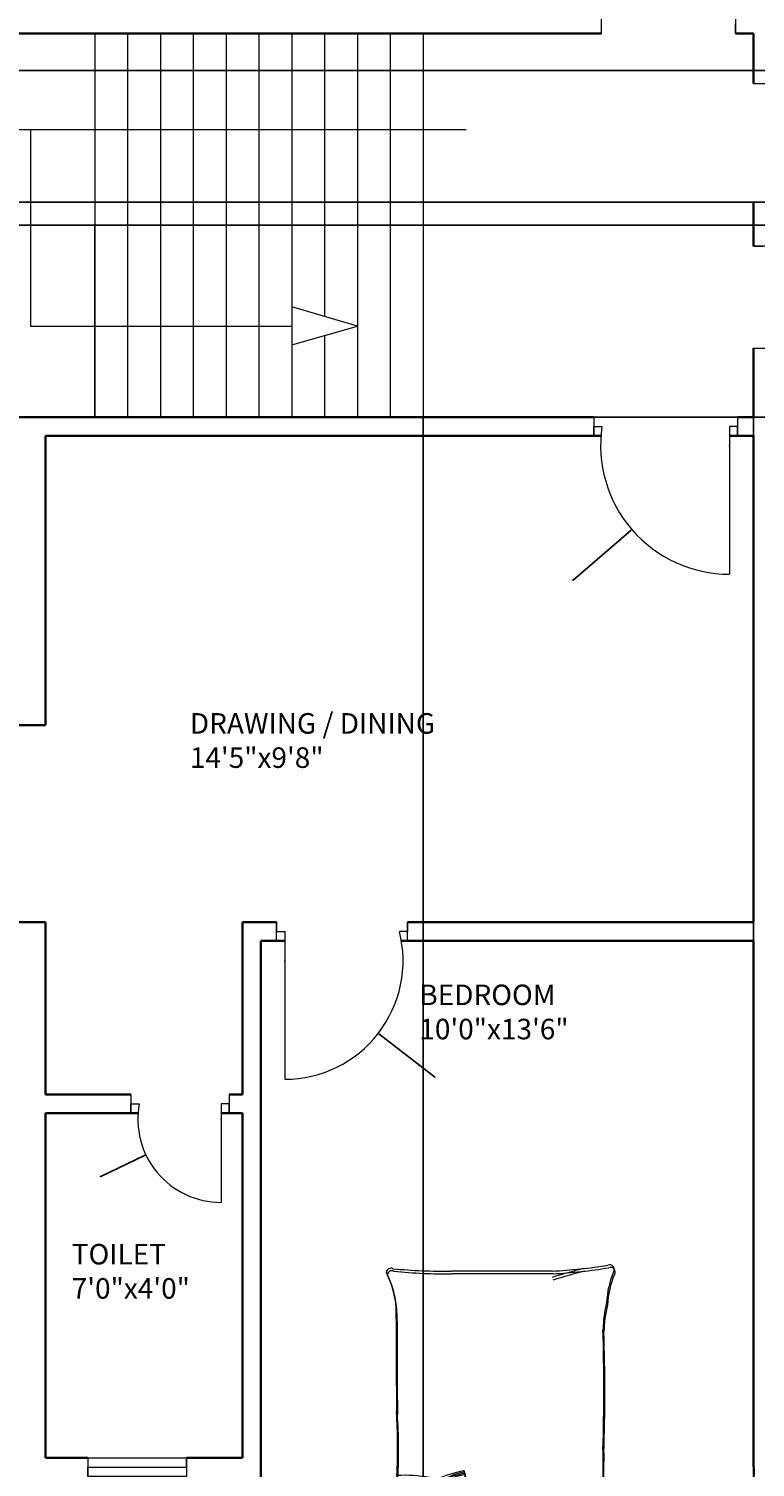
# Model space of a CAD drawing. Units: inches. Extents: x 1937 to 2996, y 1402 to 2323.
# Tile 4 of 10: x 2466 to 2643, y 1594 to 1944. Entities that reach past the tile are written whole.
import ezdxf

# ---------------------------------------------------------------- set-up
doc = ezdxf.new("R2010")
doc.units = ezdxf.units.IN
for name, color, linetype, lineweight in [('A-ANNO-DIMS', 2, 'Continuous', 18), ('A-AREA-IDEN', 7, 'Continuous', 18), ('A-DOOR', 11, 'Continuous', 18), ('A-FLOR-STRS', 81, 'Continuous', 18), ('A-FURN', 8, 'Continuous', 13), ('A-GLAZ', 141, 'Continuous', 18), ('A-WALL', 7, 'Continuous', 35)]:
    doc.layers.add(name, color=color, linetype=linetype, lineweight=lineweight)
doc.styles.get("Standard").update_dxf_attribs({"font": 'arial.ttf'})
doc.dimstyles.get("Standard").update_dxf_attribs({"dimtxt": 0.18, "dimasz": 0.18, "dimexe": 0.18, "dimexo": 0.0625, "dimgap": 0.09, "dimtad": 0, "dimtih": 1, "dimtoh": 1, "dimdec": 4, "dimzin": 0, "dimdsep": 46, "dimtxsty": 'Standard', "dimcen": 0.09, "dimadec": 0, "dimazin": 0, "dimtfac": 1, "dimtdec": 4, "dimtofl": 0, "dimtmove": 0, "dimatfit": 3, "dimfxl": 1, "dimtolj": 1, "dimtzin": 0, "dimarcsym": 0})

# ---------------------------------------------------------------- blocks, each defined once
blk = doc.blocks.new('BED-DOUBLE')
for p, q in [((-24.01, -18.11), (-24.01, 0)), ((-24.01, -18.11), (-24.01, 0)), ((-24.01, 0), (24.01, 0)), ((23.78, 0), (23.78, -26.61)), ((23.78, 0), (23.78, -26.61)), ((24.01, 0), (24.01, -0.64)), ((-24.01, -1.53), (23.78, -1.53)), ((-24.01, -1.53), (23.78, -1.53)), ((-23.78, -18.75), (-23.78, -0.64)), ((-23.78, -18.75), (-23.78, -0.64)), ((-23.78, -2.17), (24.01, -2.17)), ((-23.78, -2.17), (24.01, -2.17)), ((-23.59, -3.34), (-19.3, -3.01)), ((-23.59, -3.34), (-19.31, -3.01)), ((-23.59, -3.32), (-23.01, -6.5)), ((-23.59, -3.32), (-23.01, -6.5)), ((-19.31, -3.01), (-19.2, -3.03)), ((-19.3, -3.01), (-19.2, -3.03)), ((-19.2, -3.03), (-15.38, -3.32)), ((-19.2, -3.03), (-15.38, -3.32)), ((-15.38, -3.32), (-9.88, -4.33)), ((-15.38, -3.32), (-9.88, -4.33)), ((-12.63, -3.75), (-10.61, -3.03)), ((-12.63, -3.75), (-10.61, -3.03)), ((-10.61, -3.03), (-7.71, -2.3)), ((-10.61, -3.03), (-7.71, -2.3)), ((-10.38, -3.67), (-7.49, -2.94)), ((-10.38, -3.67), (-7.49, -2.94)), ((-7.71, -2.3), (-7.39, -2.3)), ((-7.71, -2.3), (-7.39, -2.3)), ((-7.49, -2.94), (-7.16, -2.94)), ((-7.49, -2.94), (-7.16, -2.94)), ((-7.39, -2.3), (-2.95, -2.45)), ((-7.39, -2.3), (-2.95, -2.45)), ((-7.16, -2.94), (-2.72, -3.09)), ((-7.16, -2.94), (-2.72, -3.09)), ((-2.95, -2.45), (-1.5, -1.87)), ((-2.95, -2.45), (-1.5, -1.87)), ((-2.72, -3.09), (-1.27, -2.51)), ((-2.72, -3.09), (-1.27, -2.51)), ((-1.5, -1.87), (-0.92, -7.22)), ((-1.5, -1.87), (-0.92, -7.22)), ((-1.27, -2.51), (-0.7, -7.86)), ((-1.27, -2.51), (-0.7, -7.86)), ((0.49, -2.49), (0.25, -7.87)), ((0.49, -2.49), (0.25, -7.87)), ((0.72, -3.13), (0.48, -8.51)), ((0.72, -3.13), (0.48, -8.51)), ((1.97, -2.98), (0.49, -2.49)), ((1.97, -2.98), (0.49, -2.49)), ((2.2, -3.62), (0.72, -3.13)), ((2.2, -3.62), (0.72, -3.13)), ((6.4, -2.56), (1.97, -2.98)), ((6.4, -2.56), (1.97, -2.98)), ((6.63, -3.2), (2.2, -3.62)), ((6.63, -3.2), (2.2, -3.62)), ((6.72, -2.54), (6.4, -2.56)), ((6.72, -2.54), (6.4, -2.56)), ((6.95, -3.18), (6.63, -3.2)), ((6.95, -3.18), (6.63, -3.2)), ((9.65, -3.08), (6.72, -2.54)), ((9.65, -3.08), (6.72, -2.54)), ((9.88, -3.72), (6.95, -3.18)), ((9.88, -3.72), (6.95, -3.18)), ((14.43, -3.07), (9.01, -4.42)), ((14.43, -3.07), (9.01, -4.42)), ((11.72, -3.67), (9.65, -3.08)), ((11.72, -3.67), (9.65, -3.08)), ((18.23, -2.54), (14.43, -3.07)), ((18.23, -2.54), (14.43, -3.07)), ((18.46, -3.18), (14.66, -3.71)), ((18.46, -3.18), (14.66, -3.71)), ((22.63, -2.56), (17.23, -2.46)), ((17.23, -2.46), (18.23, -2.54)), ((22.63, -2.56), (17.23, -2.46)), ((17.23, -2.46), (18.23, -2.54)), ((22.86, -3.2), (17.45, -3.1)), ((17.45, -3.1), (18.46, -3.18)), ((22.86, -3.2), (17.45, -3.1)), ((17.45, -3.1), (18.46, -3.18)), ((22.63, -2.56), (22.25, -5.77)), ((22.63, -2.56), (22.25, -5.77)), ((22.86, -3.2), (22.48, -6.41)), ((22.86, -3.2), (22.48, -6.41)), ((24.01, -0.64), (24.01, -27.25)), ((24.01, -0.64), (24.01, -27.25)), ((-23.01, -6.5), (-23.45, -9.1)), ((-23.01, -6.5), (-23.45, -9.1)), ((-23.36, -3.98), (-19.08, -3.65)), ((-23.36, -3.98), (-19.08, -3.65)), ((-23.36, -3.96), (-22.78, -7.14)), ((-23.36, -3.96), (-22.78, -7.14)), ((-22.43, -8.96), (-21.42, -6.21)), ((-22.43, -8.96), (-21.42, -6.21)), ((-22.21, -9.59), (-21.19, -6.85)), ((-22.2, -9.59), (-21.19, -6.85)), ((-19.08, -3.65), (-18.97, -3.67)), ((-19.08, -3.65), (-18.97, -3.67)), ((-18.97, -3.67), (-15.15, -3.96)), ((-18.97, -3.67), (-15.15, -3.96)), ((-15.15, -3.96), (-9.65, -4.97)), ((-15.15, -3.96), (-9.65, -4.97)), ((-12.4, -4.39), (-10.38, -3.67)), ((-12.4, -4.39), (-10.38, -3.67)), ((14.66, -3.71), (9.24, -5.06)), ((14.66, -3.71), (9.24, -5.06)), ((11.94, -4.31), (9.88, -3.72)), ((11.94, -4.31), (9.88, -3.72)), ((21.83, -8.26), (20.64, -5.58)), ((21.82, -8.26), (20.64, -5.58)), ((22.05, -8.9), (20.87, -6.22)), ((22.05, -8.9), (20.87, -6.22)), ((22.25, -5.77), (22.84, -8.34)), ((22.25, -5.77), (22.84, -8.34)), ((22.48, -6.41), (23.07, -8.98)), ((22.48, -6.41), (23.07, -8.98)), ((-23.45, -9.1), (-22.87, -10.11)), ((-23.45, -9.1), (-22.87, -10.11)), ((-22.78, -7.14), (-23.22, -9.74)), ((-22.78, -7.14), (-23.22, -9.74)), ((-23.22, -9.74), (-22.64, -10.75)), ((-23.22, -9.74), (-22.64, -10.75)), ((-23.01, -12.57), (-22.43, -8.96)), ((-23.01, -12.57), (-22.43, -8.96)), ((-22.78, -13.21), (-22.2, -9.59)), ((-22.78, -13.21), (-22.21, -9.59)), ((-0.92, -7.22), (-0.35, -10.4)), ((-0.92, -7.22), (-0.35, -10.4)), ((-0.7, -7.86), (-0.12, -11.04)), ((-0.7, -7.86), (-0.12, -11.04)), ((-0.35, -10.4), (-0.35, -11.7)), ((-0.35, -10.4), (-0.35, -11.7)), ((0.25, -7.87), (-0.13, -11.08)), ((0.25, -7.87), (-0.13, -11.08)), ((0.48, -8.51), (0.1, -11.72)), ((0.48, -8.51), (0.1, -11.72)), ((22.63, -11.83), (21.82, -8.26)), ((22.63, -11.83), (21.83, -8.26)), ((22.86, -12.47), (22.05, -8.9)), ((22.86, -12.47), (22.05, -8.9)), ((22.84, -8.34), (22.33, -9.38)), ((22.84, -8.34), (22.33, -9.38)), ((23.07, -8.98), (22.56, -10.02)), ((23.07, -8.98), (22.56, -10.02)), ((-22.72, -14.16), (-23.01, -12.57)), ((-22.72, -14.16), (-23.01, -12.57)), ((-22.49, -14.8), (-22.78, -13.21)), ((-22.49, -14.8), (-22.78, -13.21)), ((-0.35, -11.7), (-0.92, -13.58)), ((-0.35, -11.7), (-0.92, -13.58)), ((-0.92, -13.58), (-0.92, -16.26)), ((-0.92, -13.58), (-0.92, -16.26)), ((-0.12, -12.34), (-0.7, -14.22)), ((-0.12, -12.34), (-0.7, -14.22)), ((-0.13, -11.08), (-0.05, -12.38)), ((-0.13, -11.08), (-0.05, -12.38)), ((-0.12, -11.04), (-0.12, -12.34)), ((-0.12, -11.04), (-0.12, -12.34)), ((-0.05, -12.38), (0.65, -14.22)), ((-0.05, -12.38), (0.65, -14.22)), ((0.1, -11.72), (0.18, -13.02)), ((0.1, -11.72), (0.18, -13.02)), ((0.18, -13.02), (0.87, -14.86)), ((0.18, -13.02), (0.87, -14.86)), ((22.44, -13.43), (22.63, -11.83)), ((22.44, -13.43), (22.63, -11.83)), ((23.21, -16.57), (22.44, -13.43)), ((23.21, -16.57), (22.44, -13.43)), ((22.67, -14.07), (22.86, -12.47)), ((22.67, -14.07), (22.86, -12.47)), ((-23.3, -17.34), (-22.72, -14.16)), ((-23.3, -17.34), (-22.72, -14.16)), ((-18.2, -16.62), (-23.3, -17.34)), ((-18.2, -16.62), (-23.3, -17.34)), ((-23.07, -17.98), (-22.49, -14.8)), ((-23.07, -17.98), (-22.49, -14.8)), ((-17.98, -17.26), (-23.07, -17.98)), ((-17.98, -17.26), (-23.07, -17.98)), ((-21.1, -15.63), (-17.07, -16.3)), ((-21.1, -15.63), (-17.07, -16.3)), ((-20.87, -16.27), (-16.84, -16.93)), ((-20.87, -16.27), (-16.84, -16.93)), ((-17.07, -16.3), (-18.2, -16.62)), ((-17.07, -16.3), (-18.2, -16.62)), ((-16.84, -16.93), (-17.98, -17.26)), ((-16.84, -16.93), (-17.98, -17.26)), ((-17.07, -16.3), (-10.06, -16.73)), ((-17.07, -16.3), (-10.06, -16.73)), ((-16.84, -16.93), (-9.83, -17.37)), ((-16.84, -16.93), (-9.83, -17.37)), ((-10.06, -16.73), (-8.1, -16.17)), ((-10.06, -16.73), (-8.1, -16.17)), ((-9.83, -17.37), (-7.87, -16.81)), ((-9.83, -17.37), (-7.87, -16.81)), ((-8.1, -16.17), (-2.97, -16.57)), ((-8.1, -16.17), (-2.97, -16.57)), ((-7.87, -16.81), (-2.74, -17.21)), ((-7.87, -16.81), (-2.74, -17.21)), ((-3.38, -16.26), (-6.53, -15.17)), ((-3.38, -16.26), (-6.53, -15.17)), ((-3.15, -16.9), (-6.3, -15.81)), ((-3.15, -16.9), (-6.3, -15.81)), ((-0.92, -16.26), (-3.38, -16.26)), ((-0.92, -16.26), (-3.38, -16.26)), ((-0.7, -16.9), (-3.15, -16.9)), ((-0.7, -16.9), (-3.15, -16.9)), ((-0.7, -14.22), (-0.7, -16.9)), ((-0.7, -14.22), (-0.7, -16.9)), ((0.65, -14.22), (0.81, -16.89)), ((0.65, -14.22), (0.81, -16.89)), ((0.81, -16.89), (3.27, -16.74)), ((0.81, -16.89), (3.27, -16.74)), ((0.87, -14.86), (1.04, -17.53)), ((0.87, -14.86), (1.04, -17.53)), ((1.04, -17.53), (3.49, -17.38)), ((1.04, -17.53), (3.49, -17.38)), ((2.77, -17.38), (6.97, -23.88)), ((2.77, -17.38), (6.96, -23.88)), ((3.27, -16.74), (6.34, -15.45)), ((3.27, -16.74), (6.34, -15.45)), ((3.49, -17.38), (6.56, -16.09)), ((3.49, -17.38), (6.56, -16.09)), ((13.16, -20.32), (4.82, -17.38)), ((13.16, -20.32), (4.82, -17.38)), ((5.08, -15.63), (9.11, -16.3)), ((5.08, -15.63), (9.11, -16.3)), ((5.31, -16.27), (9.34, -16.93)), ((5.31, -16.27), (9.34, -16.93)), ((9.11, -16.3), (16.12, -16.73)), ((9.11, -16.3), (16.12, -16.73)), ((9.34, -16.93), (16.35, -17.37)), ((9.34, -16.93), (16.35, -17.37)), ((16.12, -16.73), (18.08, -16.17)), ((16.12, -16.73), (18.08, -16.17)), ((16.35, -17.37), (18.31, -16.81)), ((16.35, -17.37), (18.31, -16.81)), ((18.08, -16.17), (23.21, -16.57)), ((18.08, -16.17), (23.21, -16.57)), ((18.31, -16.81), (23.44, -17.21)), ((18.31, -16.81), (23.44, -17.21)), ((23.44, -17.21), (22.67, -14.07)), ((23.44, -17.21), (22.67, -14.07)), ((3, -18.02), (7.19, -24.52)), ((3, -18.02), (7.19, -24.52)), ((13.39, -20.96), (5.05, -18.02)), ((13.39, -20.96), (5.05, -18.02)), ((18.74, -22.33), (13.16, -20.32)), ((18.74, -22.33), (13.16, -20.32)), ((18.96, -22.97), (13.39, -20.96)), ((18.96, -22.97), (13.39, -20.96)), ((6.96, -23.88), (8.67, -28.37)), ((6.97, -23.88), (8.67, -28.37)), ((7.19, -24.52), (8.9, -29)), ((7.19, -24.52), (8.9, -29)), ((21.68, -24.5), (18.74, -22.33)), ((21.68, -24.5), (18.74, -22.33)), ((21.91, -25.13), (18.96, -22.97)), ((21.91, -25.13), (18.96, -22.97)), ((25.38, -27.75), (21.68, -24.5)), ((25.38, -27.75), (21.68, -24.5)), ((25.61, -28.39), (21.91, -25.13)), ((25.61, -28.39), (21.91, -25.13)), ((23.85, -28.37), (25.38, -27.75)), ((23.85, -28.37), (25.38, -27.75)), ((25.46, -29.49), (25.38, -27.75, 3.87)), ((25.46, -29.49), (25.38, -27.75, 3.87)), ((8.67, -28.37), (8.98, -30.38)), ((8.67, -28.37), (8.98, -30.38)), ((8.9, -29), (9.21, -31.02)), ((8.9, -29), (9.21, -31.02)), ((8.98, -30.38), (11.46, -29.76)), ((8.98, -30.38), (11.46, -29.76)), ((9.21, -31.02), (11.68, -30.4)), ((9.21, -31.02), (11.68, -30.4)), ((11.46, -29.76), (13.47, -28.83)), ((11.46, -29.76), (13.47, -28.83)), ((11.68, -30.4), (13.7, -29.47)), ((11.68, -30.4), (13.7, -29.47)), ((13.47, -28.83), (16.88, -28.37)), ((13.47, -28.83), (16.88, -28.37)), ((13.7, -29.47), (17.11, -29)), ((13.7, -29.47), (17.1, -29)), ((16.88, -28.37), (20.75, -28.06)), ((16.88, -28.37), (20.75, -28.06)), ((17.1, -29), (20.98, -28.69)), ((17.11, -29), (20.98, -28.69)), ((20.75, -28.06), (23.85, -28.37)), ((20.75, -28.06), (23.85, -28.37)), ((20.98, -28.69), (24.07, -29)), ((20.98, -28.69), (24.07, -29)), ((24.07, -29), (25.61, -28.39)), ((24.07, -29), (25.61, -28.39)), ((25.69, -30.13), (25.61, -28.39, 3.87)), ((25.69, -30.13), (25.61, -28.39, 3.87)), ((-12.42, -79.25), (12.19, -79.25)), ((-12.42, -79.25), (12.19, -79.25)), ((-12.19, -79.88), (12.42, -79.88)), ((-12.19, -79.88), (12.42, -79.88))]:
    blk.add_line(p, q)
for centre, radius, start, end in [((-6.13, -182.05), 164.97, 86.0865, 96.7821), ((-6.13, -182.05), 164.97, 86.0865, 96.7821), ((57.68, -20.1), 83.31, 178.7218, 185.604), ((57.68, -20.1), 83.31, 178.7218, 185.604), ((57.91, -20.74), 83.31, 178.7218, 185.604), ((57.91, -20.74), 83.31, 178.7218, 185.604), ((-5.9, -182.69), 164.97, 86.0865, 96.7821), ((-5.9, -182.69), 164.97, 86.0865, 96.7821), ((-9.73, -156.32), 129.02, 81.7845, 96.9006), ((-9.73, -156.32), 129.02, 81.7845, 96.9006), ((-9.5, -156.96), 129.02, 81.7845, 96.9006), ((-9.5, -156.96), 129.02, 81.7845, 96.9006), ((-194.79, -31.17), 170.11, 358.4762, 1.0082), ((-194.79, -31.17), 170.11, 358.4762, 1.0082), ((-194.56, -31.81), 170.11, 358.4762, 1.0082), ((-194.56, -31.81), 170.11, 358.4762, 1.0082), ((9.15, -30.44), 0.185, 160.2464, 271.1377), ((9.15, -30.44), 0.185, 160.2464, 271.1377), ((3.67, -1.48), 29.65, 280.6617, 289.8806), ((3.67, -1.48), 29.65, 280.6617, 289.8806), ((9.38, -31.08), 0.185, 160.2464, 271.1377), ((9.38, -31.08), 0.185, 160.2464, 271.1377), ((3.9, -2.12), 29.65, 280.6617, 289.8806), ((3.9, -2.12), 29.65, 280.6617, 289.8806), ((16.26, -35.07), 6.22, 78.6608, 113.7384), ((16.26, -35.07), 6.22, 78.6608, 113.7384), ((16.49, -35.71), 6.22, 78.6608, 113.7384), ((16.49, -35.71), 6.22, 78.6608, 113.7384), ((23.84, 6.66), 36.18, 259.8763, 272.5657), ((23.84, 6.66), 36.18, 259.8763, 272.5657), ((24.07, 6.02), 36.18, 259.8763, 272.5657), ((24.07, 6.02), 36.18, 259.8763, 272.5657), ((154.78, -36.32), 129.5, 176.9791, 183.8365), ((154.78, -36.32), 129.5, 176.9791, 183.8365), ((155.01, -36.95), 129.5, 176.9791, 183.8365), ((155.01, -36.95), 129.5, 176.9791, 183.8365), ((457.34, -50.61), 482.31, 178.2277, 181.7185), ((457.34, -50.61), 482.31, 178.2277, 181.7185), ((457.57, -51.25), 482.31, 178.2277, 181.7185), ((457.57, -51.25), 482.31, 178.2277, 181.7185), ((-4536.23, -67.82), 4561.86, 0.00217, 0.28689), ((-4536.23, -67.82), 4561.86, 0.00217, 0.28689), ((-4536, -68.46), 4561.86, 0.00217, 0.28689), ((-4536, -68.46), 4561.86, 0.00217, 0.28689), ((-54.38, -64.52), 29.63, 346.0648, 358.9113), ((-54.38, -64.52), 29.63, 346.0648, 358.9113), ((-54.16, -65.15), 29.63, 346.0648, 358.9113), ((-54.16, -65.15), 29.63, 346.0648, 358.9113), ((48.67, -68.67), 23.07, 177.4714, 206.4681), ((48.67, -68.67), 23.07, 177.4714, 206.4681), ((48.9, -69.31), 23.07, 177.4714, 206.4681), ((48.9, -69.31), 23.07, 177.4714, 206.4681), ((-49.14, -70.28), 23.56, 337.9751, 356.652), ((-49.14, -70.28), 23.56, 337.9751, 356.652), ((-48.92, -70.91), 23.56, 337.9751, 356.652), ((-48.92, -70.91), 23.56, 337.9751, 356.652), ((-26.4, -79.72), 1.09, 146.1736, 293.4781), ((-26.4, -79.72), 1.09, 146.1736, 293.4781), ((-26.17, -80.36), 1.09, 146.1736, 293.4781), ((-26.17, -80.36), 1.09, 146.1736, 293.4781), ((-6.06, -200.84), 121.76, 92.9958, 99.4091), ((-6.06, -200.84), 121.76, 92.9958, 99.4091), ((-5.83, -201.48), 121.76, 92.9958, 99.4091), ((-5.83, -201.48), 121.76, 92.9958, 99.4091), ((-44.71, 23.71), 106.46, 283.3832, 287.7053), ((-44.71, 23.71), 106.46, 283.3832, 287.7053), ((-44.48, 23.07), 106.46, 283.3832, 287.7053), ((-44.48, 23.07), 106.46, 283.3832, 287.7053), ((13.67, -212.28), 133.04, 84.4998, 90.6351), ((13.67, -212.28), 133.04, 84.4998, 90.6351), ((13.9, -212.92), 133.04, 84.4998, 90.6351), ((13.9, -212.92), 133.04, 84.4998, 90.6351), ((26.93, -78.87), 1.1, 242.6588, 356.02), ((26.93, -78.87), 1.1, 242.6588, 356.02), ((27.15, -79.51), 1.1, 242.6588, 356.02), ((27.15, -79.51), 1.1, 242.6588, 356.02)]:
    blk.add_arc(centre, radius, start, end)
blk = doc.blocks.new('WINDOW-24IN')
for p, q in [((0, -2.25), (0, 2.25)), ((0, 2.25), (0, 0)), ((24, 2.25), (0, 2.25)), ((0, 0), (24, 0)), ((24, -2.25), (24, 2.25)), ((24, 0), (24, -2.25)), ((0, -2.25), (24, -2.25))]:
    blk.add_line(p, q)
blk = doc.blocks.new('*D23')
at = {"layer": 'A-ANNO-DIMS', "color": 0, "lineweight": -2, "transparency": 16777216}
for p, q in [((2010.65, 1769.24), (2010.65, 1508.98)), ((2924.15, 1769.24), (2924.15, 1508.98)), ((2010.83, 1509.16), (2467, 1509.16)), ((2923.97, 1509.16), (2467.79, 1509.16))]:
    blk.add_line(p, q, dxfattribs=at)
at = {"layer": 'A-ANNO-DIMS', "color": 0, "transparency": 16777216}
for points in [[(2010.83, 1509.19), (2010.83, 1509.13), (2010.65, 1509.16)], [(2923.97, 1509.19), (2923.97, 1509.13), (2924.15, 1509.16)]]:
    blk.add_solid(points, dxfattribs=at)
at = {"layer": 'Defpoints', "color": 0, "transparency": 16777216}
for p in [(2010.65, 1769.31), (2924.15, 1769.31), (2924.15, 1509.16)]:
    blk.add_point(p, dxfattribs=at)
at = {"layer": 'A-ANNO-DIMS', "color": 0, "transparency": 16777216, "insert": (2467.4, 1509.16), "char_height": 0.18, "attachment_point": 5}
blk.add_mtext('\\A1;913.5', dxfattribs=at)
blk = doc.blocks.new('*D34')
at = {"layer": 'A-ANNO-DIMS', "color": 0, "lineweight": -2, "transparency": 16777216}
for p, q in [((2350.61, 1849.24), (2350.61, 1508.98)), ((2561.65, 1849.24), (2561.65, 1508.98)), ((2350.79, 1509.16), (2455.66, 1509.16)), ((2561.47, 1509.16), (2456.59, 1509.16))]:
    blk.add_line(p, q, dxfattribs=at)
at = {"layer": 'A-ANNO-DIMS', "color": 0, "transparency": 16777216}
for points in [[(2350.79, 1509.19), (2350.79, 1509.13), (2350.61, 1509.16)], [(2561.47, 1509.19), (2561.47, 1509.13), (2561.65, 1509.16)]]:
    blk.add_solid(points, dxfattribs=at)
at = {"layer": 'Defpoints', "color": 0, "transparency": 16777216}
for p in [(2350.61, 1849.31), (2561.65, 1849.31), (2561.65, 1509.16)]:
    blk.add_point(p, dxfattribs=at)
at = {"layer": 'A-ANNO-DIMS', "color": 0, "transparency": 16777216, "insert": (2456.13, 1509.16), "char_height": 0.18, "attachment_point": 5}
blk.add_mtext('\\A1;211.04', dxfattribs=at)
blk = doc.blocks.new('*D35')
at = {"layer": 'A-ANNO-DIMS', "color": 0, "lineweight": -2, "transparency": 16777216}
for p, q in [((2561.65, 1849.24), (2561.65, 1508.98)), ((2642.15, 1849.24), (2642.15, 1508.98)), ((2561.83, 1509.16), (2601.57, 1509.16)), ((2641.97, 1509.16), (2602.22, 1509.16))]:
    blk.add_line(p, q, dxfattribs=at)
at = {"layer": 'A-ANNO-DIMS', "color": 0, "transparency": 16777216}
for points in [[(2561.83, 1509.19), (2561.83, 1509.13), (2561.65, 1509.16)], [(2641.97, 1509.19), (2641.97, 1509.13), (2642.15, 1509.16)]]:
    blk.add_solid(points, dxfattribs=at)
at = {"layer": 'Defpoints', "color": 0, "transparency": 16777216}
for p in [(2561.65, 1849.31), (2642.15, 1849.31), (2642.15, 1509.16)]:
    blk.add_point(p, dxfattribs=at)
at = {"layer": 'A-ANNO-DIMS', "color": 0, "transparency": 16777216, "insert": (2601.9, 1509.16), "char_height": 0.18, "attachment_point": 5}
blk.add_mtext('\\A1;80.5', dxfattribs=at)
blk = doc.blocks.new('*D37')
at = {"layer": 'A-ANNO-DIMS', "color": 0, "lineweight": -2, "transparency": 16777216}
for p, q in [((2455.84, 1896.06), (2970.48, 1896.06)), ((2970.3, 1895.88), (2970.3, 1872.86)), ((2970.3, 1849.49), (2970.3, 1872.5)), ((2455.84, 1849.31), (2970.48, 1849.31))]:
    blk.add_line(p, q, dxfattribs=at)
at = {"layer": 'A-ANNO-DIMS', "color": 0, "transparency": 16777216}
for points in [[(2970.27, 1895.88), (2970.33, 1895.88), (2970.3, 1896.06)], [(2970.27, 1849.49), (2970.33, 1849.49), (2970.3, 1849.31)]]:
    blk.add_solid(points, dxfattribs=at)
at = {"layer": 'Defpoints', "color": 0, "transparency": 16777216}
for p in [(2455.77, 1896.06), (2455.77, 1849.31), (2970.3, 1849.31)]:
    blk.add_point(p, dxfattribs=at)
at = {"layer": 'A-ANNO-DIMS', "color": 0, "transparency": 16777216, "insert": (2970.3, 1872.68), "char_height": 0.18, "attachment_point": 5}
blk.add_mtext('\\A1;46.75', dxfattribs=at)
blk = doc.blocks.new('*D50')
at = {"layer": 'A-ANNO-DIMS', "color": 0, "lineweight": -2, "transparency": 16777216}
for p, q in [((2292.71, 1933.76), (2970.48, 1933.76)), ((2970.3, 1933.58), (2970.3, 1917.9)), ((2970.3, 1901.85), (2970.3, 1917.53)), ((2292.71, 1901.67), (2970.48, 1901.67))]:
    blk.add_line(p, q, dxfattribs=at)
at = {"layer": 'A-ANNO-DIMS', "color": 0, "transparency": 16777216}
for points in [[(2970.27, 1933.58), (2970.33, 1933.58), (2970.3, 1933.76)], [(2970.27, 1901.85), (2970.33, 1901.85), (2970.3, 1901.67)]]:
    blk.add_solid(points, dxfattribs=at)
at = {"layer": 'Defpoints', "color": 0, "transparency": 16777216}
for p in [(2292.65, 1933.76), (2970.3, 1933.76), (2292.65, 1901.67)]:
    blk.add_point(p, dxfattribs=at)
at = {"layer": 'A-ANNO-DIMS', "color": 0, "transparency": 16777216, "insert": (2970.3, 1917.71), "char_height": 0.18, "attachment_point": 5}
blk.add_mtext('\\A1;32.085', dxfattribs=at)
blk = doc.blocks.new('*D56')
at = {"layer": 'A-ANNO-DIMS', "color": 0, "lineweight": -2, "transparency": 16777216}
for p, q in [((2636.21, 1842.45), (2636.39, 1842.45)), ((2636.3, 1842.36), (2636.3, 1842.54)), ((2598.27, 1809.64), (2612.4, 1821.83)), ((2598.09, 1809.64), (2598.27, 1809.64))]:
    blk.add_line(p, q, dxfattribs=at)
at = {"layer": 'A-ANNO-DIMS', "color": 0, "transparency": 16777216}
blk.add_solid([(2612.38, 1821.85), (2612.42, 1821.8), (2612.53, 1821.94)], dxfattribs=at)
at = {"layer": 'Defpoints', "color": 0, "transparency": 16777216}
for p in [(2636.3, 1842.45), (2612.53, 1821.94)]:
    blk.add_point(p, dxfattribs=at)
at = {"layer": 'A-ANNO-DIMS', "color": 0, "transparency": 16777216, "insert": (2597.54, 1809.64), "char_height": 0.18, "attachment_point": 5}
blk.add_mtext('\\A1;R31.394', dxfattribs=at)
blk = doc.blocks.new('*D64')
at = {"layer": 'A-ANNO-DIMS', "color": 0, "lineweight": -2, "transparency": 16777216}
for p, q in [((2527.87, 1716.88), (2528.05, 1716.88)), ((2527.96, 1716.79), (2527.96, 1716.97)), ((2564.41, 1688.62), (2550.88, 1699.11)), ((2564.59, 1688.62), (2564.41, 1688.62))]:
    blk.add_line(p, q, dxfattribs=at)
at = {"layer": 'A-ANNO-DIMS', "color": 0, "transparency": 16777216}
blk.add_solid([(2550.9, 1699.13), (2550.86, 1699.08), (2550.74, 1699.22)], dxfattribs=at)
at = {"layer": 'Defpoints', "color": 0, "transparency": 16777216}
for p in [(2527.96, 1716.88), (2550.74, 1699.22)]:
    blk.add_point(p, dxfattribs=at)
at = {"layer": 'A-ANNO-DIMS', "color": 0, "transparency": 16777216, "insert": (2565.14, 1688.62), "char_height": 0.18, "attachment_point": 5}
blk.add_mtext('\\A1;R28.823', dxfattribs=at)
blk = doc.blocks.new('*D86')
at = {"layer": 'A-ANNO-DIMS', "color": 0, "lineweight": -2, "transparency": 16777216}
for p, q in [((2512.36, 1678.36), (2512.54, 1678.36)), ((2512.45, 1678.27), (2512.45, 1678.45)), ((2483.12, 1664.39), (2493.96, 1669.55)), ((2482.94, 1664.39), (2483.12, 1664.39))]:
    blk.add_line(p, q, dxfattribs=at)
at = {"layer": 'A-ANNO-DIMS', "color": 0, "transparency": 16777216}
blk.add_solid([(2493.94, 1669.58), (2493.97, 1669.52), (2494.12, 1669.63)], dxfattribs=at)
at = {"layer": 'Defpoints', "color": 0, "transparency": 16777216}
for p in [(2512.45, 1678.36), (2494.12, 1669.63)]:
    blk.add_point(p, dxfattribs=at)
at = {"layer": 'A-ANNO-DIMS', "color": 0, "transparency": 16777216, "insert": (2482.39, 1664.39), "char_height": 0.18, "attachment_point": 5}
blk.add_mtext('\\A1;R20.303', dxfattribs=at)

msp = doc.modelspace()

# ---------------------------------------------------------------- linework, layer by layer
at = {"layer": 'A-DOOR'}
for p, q in [((2605.163, 1942.8061), (2605.163, 1947.3061)), ((2637.7727, 1947.3061), (2637.7727, 1942.8061)), ((2637.7727, 1942.8061), (2637.7727, 1945.0561)), ((2642.1473, 1930.5712), (2646.6473, 1930.5712)), ((2646.6473, 1901.7001), (2642.1473, 1901.7001)), ((2642.1473, 1901.7001), (2644.3973, 1901.7001)), ((2646.6473, 1890.9534), (2642.1473, 1890.9534)), ((2642.1473, 1890.9534), (2644.3973, 1890.9534)), ((2642.1473, 1866.1389), (2646.6473, 1866.1389)), ((2603.2509, 1849.3061), (2603.2509, 1844.8061)), ((2603.2509, 1844.8061), (2603.2509, 1847.0561)), ((2603.2509, 1847.0561), (2605.2509, 1847.0561)), ((2638.3047, 1847.0561), (2636.3047, 1847.0561)), ((2636.3047, 1847.0561), (2636.3047, 1823.0561)), ((2638.3047, 1849.3061), (2638.3047, 1844.8061)), ((2638.3047, 1844.8061), (2638.3047, 1847.0561)), ((2636.3047, 1823.0561), (2636.3047, 1811.0561)), ((2525.9612, 1721.8061), (2525.9612, 1726.3061)), ((2525.9612, 1726.3061), (2525.9612, 1724.0561)), ((2525.9612, 1724.0561), (2525.9612, 1724.0561)), ((2525.9612, 1724.0561), (2527.9612, 1724.0561)), ((2527.9612, 1724.0561), (2527.9612, 1688.0561)), ((2557.877, 1724.0561), (2555.877, 1724.0561)), ((2557.877, 1721.8061), (2557.877, 1726.3061)), ((2557.877, 1726.3061), (2557.877, 1724.0561)), ((2490.4845, 1684.3061), (2490.4845, 1679.8061)), ((2490.4845, 1679.8061), (2490.4845, 1682.0561)), ((2490.4845, 1682.0561), (2492.4845, 1682.0561)), ((2514.4482, 1682.0561), (2512.4482, 1682.0561)), ((2512.4482, 1682.0561), (2512.4482, 1658.0561)), ((2514.4482, 1684.3061), (2514.4482, 1679.8061)), ((2514.4482, 1679.8061), (2514.4482, 1682.0561))]:
    msp.add_line(p, q, dxfattribs=at)
for centre, radius, start, end in [((2636.3047, 1842.4498), 31.3936, 171.562601, 270), ((2527.9612, 1716.8796), 28.8235, 270, 14.417318), ((2512.4482, 1678.3593), 20.3032, 169.508913, 270)]:
    msp.add_arc(centre, radius, start, end, dxfattribs=at)
at = {"layer": 'A-FLOR-STRS'}
for p, q in [((2481.6473, 1942.8061), (2481.6473, 1849.3061)), ((2489.6473, 1942.8061), (2489.6473, 1849.3061)), ((2497.6473, 1942.8061), (2497.6473, 1849.3061)), ((2505.6473, 1942.8061), (2505.6473, 1849.3061)), ((2513.6473, 1942.8061), (2513.6473, 1849.3061)), ((2521.6473, 1942.8061), (2521.6473, 1849.3061)), ((2529.6473, 1942.8061), (2529.6473, 1849.3061)), ((2537.6473, 1942.8061), (2537.6473, 1873.8269)), ((2545.6473, 1942.8061), (2545.6473, 1849.3061)), ((2553.6473, 1942.8061), (2553.6473, 1849.3061)), ((2561.6473, 1942.8061), (2561.6473, 1849.3061)), ((2572.1291, 1919.2771), (2382.6104, 1919.2771)), ((2466.0021, 1919.2771), (2466.0021, 1871.4712)), ((2481.6473, 1849.3061), (2481.6473, 1896.0561)), ((2481.6473, 1896.0561), (2561.5364, 1896.0561)), ((2545.6473, 1871.4712), (2529.6473, 1876.1825)), ((2529.6473, 1876.1825), (2529.6473, 1866.9083)), ((2466.0021, 1871.4712), (2529.6473, 1871.4712)), ((2529.6473, 1866.9083), (2545.6473, 1871.4712)), ((2537.6473, 1869.1897), (2537.6473, 1849.3061))]:
    msp.add_line(p, q, dxfattribs=at)
at = {"layer": 'A-WALL'}
for p, q in [((2316.6473, 1942.8061), (2605.163, 1942.8061)), ((2637.7727, 1942.8061), (2642.1473, 1942.8061)), ((2642.1473, 1942.8061), (2642.1473, 1930.5712)), ((2642.1473, 1901.7001), (2642.1473, 1890.9534)), ((2642.1473, 1866.1389), (2642.1473, 1849.3061)), ((2316.6473, 1849.3061), (2603.2509, 1849.3061)), ((2638.3047, 1849.3061), (2642.1473, 1849.3061)), ((2469.6473, 1844.8061), (2604.9997, 1844.8061)), ((2469.6473, 1844.8061), (2469.6473, 1774.3061)), ((2636.3047, 1844.8061), (2642.1473, 1844.8061)), ((2642.1473, 1844.8061), (2642.1473, 1726.3061)), ((2461.9146, 1774.3061), (2469.6473, 1774.3061)), ((2461.8174, 1726.3061), (2469.6473, 1726.3061)), ((2469.6473, 1726.3061), (2469.6473, 1684.3061)), ((2517.6473, 1726.3061), (2517.6473, 1684.3061)), ((2517.6473, 1726.3061), (2525.9612, 1726.3061)), ((2557.877, 1726.3061), (2642.1473, 1726.3061)), ((2522.1473, 1721.8061), (2522.1473, 1595.8061)), ((2522.1473, 1721.8061), (2527.9612, 1721.8061)), ((2556.3605, 1721.8061), (2642.1473, 1721.8061)), ((2642.1473, 1721.8061), (2642.1473, 1595.8061)), ((2469.6473, 1684.3061), (2490.4845, 1684.3061)), ((2514.4482, 1684.3061), (2517.6473, 1684.3061)), ((2469.6473, 1679.8061), (2469.6473, 1595.8061)), ((2492.1967, 1679.8061), (2469.6473, 1679.8061)), ((2517.6473, 1679.8061), (2512.4482, 1679.8061)), ((2517.6473, 1595.8061), (2517.6473, 1679.8061)), ((2517.6473, 1679.8061), (2517.6473, 1595.8061)), ((2469.6473, 1595.8061), (2480.0063, 1595.8061)), ((2504.0063, 1595.8061), (2517.6473, 1595.8061)), ((2522.1473, 1559.8061), (2522.1473, 1595.8061)), ((2642.1473, 1595.8061), (2642.2867, 1591.3061))]:
    msp.add_line(p, q, dxfattribs=at)

# ---------------------------------------------------------------- block references
at = {"layer": 'A-FURN', "rotation": 180}
msp.add_blockref('BED-DOUBLE', (2580.9749, 1561.4249), dxfattribs=at)
at = {"layer": 'A-GLAZ', "extrusion": (0, 0, -1), "zscale": -1, "rotation": 180}
msp.add_blockref('WINDOW-24IN', (-2480.0063, 1593.5561), dxfattribs=at)

# ---------------------------------------------------------------- texts
at = {"layer": 'A-AREA-IDEN', "char_height": 5, "attachment_point": 1}
for s, width, insert in [('DRAWING / DINING\\P14\'5"x9\'8"', 173.749656, (2504.8295, 1777.2358)), ('BEDROOM\\P10\'0"x13\'6"', 157.491568, (2560.7483, 1711.1172)), ('TOILET\\P7\'0"x4\'0"', 181.124067, (2476.0474, 1647.9497))]:
    msp.add_mtext_dynamic_manual_height_columns(s, width=width, gutter_width=12.5, heights=[0], dxfattribs=dict(at, insert=insert))

# ---------------------------------------------------------------- dimensions: what is measured, and where the dimension line sits
at = {"layer": 'A-ANNO-DIMS'}
for base, p1, p2, override, picture, middle in [((2970.2973, 1933.7562), (2292.6473, 1901.671), (2292.6473, 1933.7562), {"dimdec": 3, "dimlfac": 1, "dimrnd": 0, "dimzin": 0, "dimdsep": 46, "dimlunit": 2}, '*D50', (2970.2973, 1917.7136)), ((2970.2973, 1849.3061), (2455.7744, 1896.0561), (2455.7744, 1849.3061), {"dimdec": 2, "dimlfac": 1, "dimrnd": 0, "dimzin": 0, "dimdsep": 46, "dimlunit": 2}, '*D37', (2970.2973, 1872.6811))]:
    dim = msp.add_linear_dim(base=base, p1=p1, p2=p2, angle=90, dimstyle='Standard', override=override, dxfattribs=at)
    dim.commit()
    dim.dimension.update_dxf_attribs({"geometry": picture, "text_midpoint": middle})
for base, p1, p2, override, picture, middle in [((2561.6473, 1509.1561), (2350.6104, 1849.3061), (2561.6473, 1849.3061), {"dimdec": 2, "dimlfac": 1, "dimrnd": 0, "dimzin": 0, "dimdsep": 46, "dimlunit": 2}, '*D34', (2456.1289, 1509.1561)), ((2642.1473, 1509.1561), (2561.6473, 1849.3061), (2642.1473, 1849.3061), {"dimdec": 1, "dimlfac": 1, "dimrnd": 0, "dimzin": 0, "dimdsep": 46, "dimlunit": 2}, '*D35', (2601.8973, 1509.1561)), ((2924.1473, 1509.1561), (2010.6473, 1769.3061), (2924.1473, 1769.3061), {"dimdec": 1, "dimlfac": 1, "dimrnd": 0, "dimzin": 0, "dimdsep": 46, "dimlunit": 2}, '*D23', (2467.3973, 1509.1561))]:
    dim = msp.add_linear_dim(base=base, p1=p1, p2=p2, dimstyle='Standard', override=override, dxfattribs=at)
    dim.commit()
    dim.dimension.update_dxf_attribs({"geometry": picture, "text_midpoint": middle})
for center, mpoint, picture, middle in [((2636.3047, 1842.4498), (2612.5333, 1821.9442), '*D56', (2597.541, 1809.6409)), ((2527.9612, 1716.87958), (2550.73896, 1699.21703), '*D64', (2565.13538, 1688.6195)), ((2512.4482, 1678.3593), (2494.1187, 1669.6274), '*D86', (2482.3912, 1664.3883))]:
    dim = msp.add_radius_dim(center=center, mpoint=mpoint, dimstyle='Standard', override={"dimdec": 3, "dimlfac": 1, "dimrnd": 0, "dimzin": 0, "dimdsep": 46, "dimlunit": 2}, dxfattribs=at)
    dim.commit()
    dim.dimension.update_dxf_attribs({"geometry": picture, "text_midpoint": middle, "dimtype": 164})

doc.saveas('drawing.dxf')
